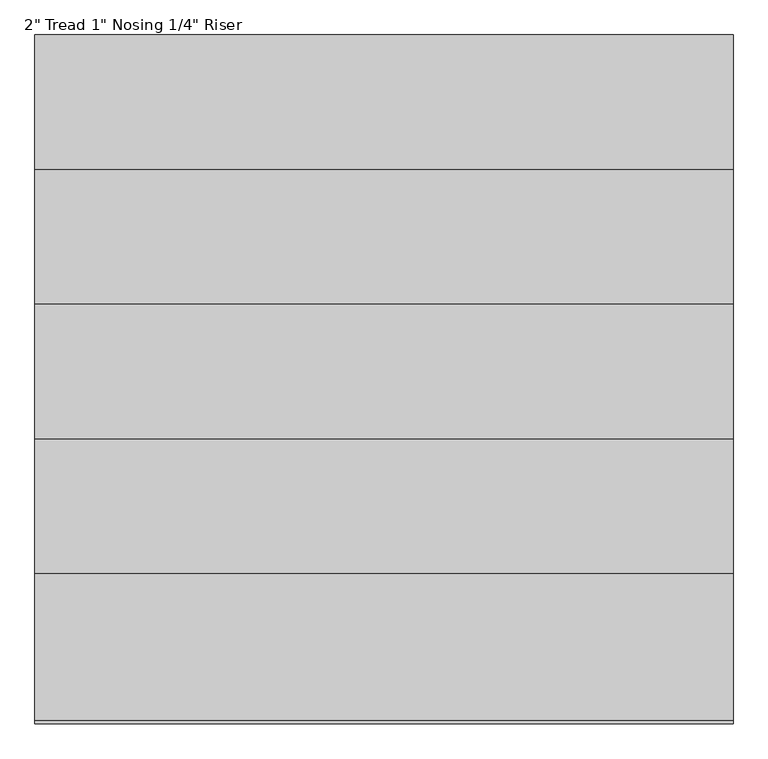
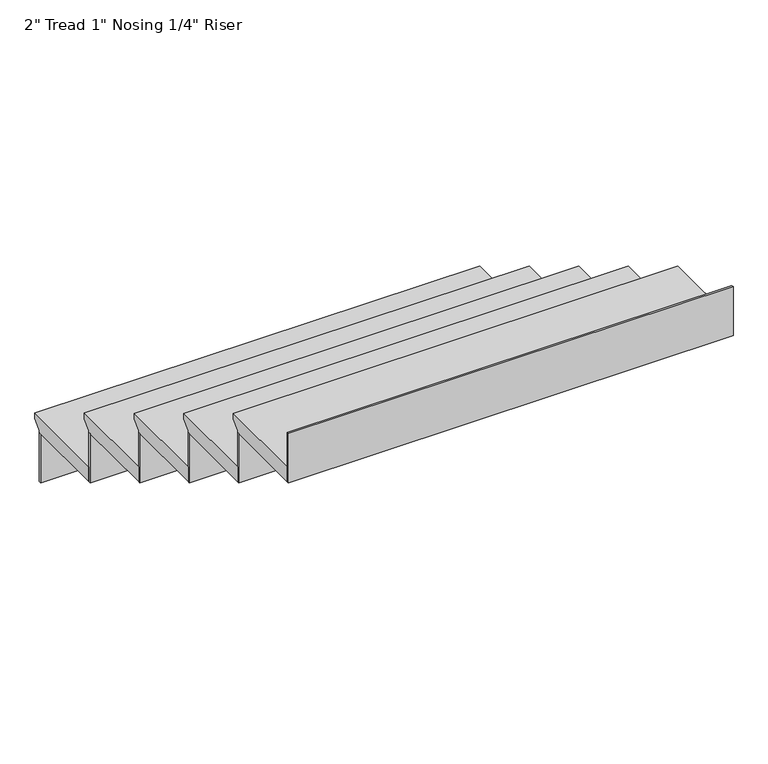
"""IFC4 building model written with IfcOpenShell, lengths in millimetres: stair flight geometry."""

from ifc_helpers import new_model, si_unit, frame, origin, place, context, project, spatial, polyline, outline, extrude, source, transform, mapped, element, save


def stair_flight_724757b1(model_context):
    return source(origin(), model_context, "Body", "SweptSolid", [
        extrude(outline(polyline([(3133.6258877, 2201.3333333), (3438.4258877, 2201.3333333), (3438.4258877, 2182.2833333), (3413.0258877, 2156.8833333), (3413.0258877, 2150.5333333), (3133.6258877, 2150.5333333), (3133.6258877, 2201.3333333)])), frame((-16853.0480019, 0.0, 0.0), z_axis=(1.0, 0.0, 0.0), x_axis=(0.0, 1.0, 0.0)), (0.0, 0.0, 1.0), 1447.8),
        extrude(outline(polyline([(-16853.0480019, 3406.6758877), (-16853.0480019, 3413.0258877), (-15405.2480019, 3413.0258877), (-15405.2480019, 3406.6758877), (-16853.0480019, 3406.6758877)])), frame((0.0, 0.0, 1981.2), z_axis=(0.0, 0.0, 1.0), x_axis=(1.0, 0.0, 0.0)), (0.0, 0.0, 1.0), 169.3333333),
        extrude(outline(polyline([(-16853.0480019, 3127.2758877), (-16853.0480019, 3133.6258877), (-15405.2480019, 3133.6258877), (-15405.2480019, 3127.2758877), (-16853.0480019, 3127.2758877)])), frame((0.0, 0.0, 2150.5333333), z_axis=(0.0, 0.0, 1.0), x_axis=(1.0, 0.0, 0.0)), (0.0, 0.0, 1.0), 169.3333333),
        extrude(outline(polyline([(2854.2258877, 2370.6666667), (3159.0258877, 2370.6666667), (3159.0258877, 2351.6166667), (3133.6258877, 2326.2166667), (3133.6258877, 2319.8666667), (2854.2258877, 2319.8666667), (2854.2258877, 2370.6666667)])), frame((-16853.0480019, 0.0, 0.0), z_axis=(1.0, 0.0, 0.0), x_axis=(0.0, 1.0, 0.0)), (0.0, 0.0, 1.0), 1447.8),
        extrude(outline(polyline([(-16853.0480019, 2847.8758877), (-16853.0480019, 2854.2258877), (-15405.2480019, 2854.2258877), (-15405.2480019, 2847.8758877), (-16853.0480019, 2847.8758877)])), frame((0.0, 0.0, 2319.8666667), z_axis=(0.0, 0.0, 1.0), x_axis=(1.0, 0.0, 0.0)), (0.0, 0.0, 1.0), 169.3333333),
        extrude(outline(polyline([(2574.8258877, 2540.0), (2879.6258877, 2540.0), (2879.6258877, 2520.95), (2854.2258877, 2495.55), (2854.2258877, 2489.2), (2574.8258877, 2489.2), (2574.8258877, 2540.0)])), frame((-16853.0480019, 0.0, 0.0), z_axis=(1.0, 0.0, 0.0), x_axis=(0.0, 1.0, 0.0)), (0.0, 0.0, 1.0), 1447.8),
        extrude(outline(polyline([(-16853.0480019, 2568.4758877), (-16853.0480019, 2574.8258877), (-15405.2480019, 2574.8258877), (-15405.2480019, 2568.4758877), (-16853.0480019, 2568.4758877)])), frame((0.0, 0.0, 2489.2), z_axis=(0.0, 0.0, 1.0), x_axis=(1.0, 0.0, 0.0)), (0.0, 0.0, 1.0), 169.3333333),
        extrude(outline(polyline([(2295.4258877, 2709.3333333), (2600.2258877, 2709.3333333), (2600.2258877, 2690.2833333), (2574.8258877, 2664.8833333), (2574.8258877, 2658.5333333), (2295.4258877, 2658.5333333), (2295.4258877, 2709.3333333)])), frame((-16853.0480019, 0.0, 0.0), z_axis=(1.0, 0.0, 0.0), x_axis=(0.0, 1.0, 0.0)), (0.0, 0.0, 1.0), 1447.8),
        extrude(outline(polyline([(-16853.0480019, 2289.0758877), (-16853.0480019, 2295.4258877), (-15405.2480019, 2295.4258877), (-15405.2480019, 2289.0758877), (-16853.0480019, 2289.0758877)])), frame((0.0, 0.0, 2658.5333333), z_axis=(0.0, 0.0, 1.0), x_axis=(1.0, 0.0, 0.0)), (0.0, 0.0, 1.0), 169.3333333),
        extrude(outline(polyline([(-16853.0480019, 2009.6758877), (-16853.0480019, 2016.0258877), (-15405.2480019, 2016.0258877), (-15405.2480019, 2009.6758877), (-16853.0480019, 2009.6758877)])), frame((0.0, 0.0, 2827.8666667), z_axis=(0.0, 0.0, 1.0), x_axis=(1.0, 0.0, 0.0)), (0.0, 0.0, 1.0), 169.3333333),
        extrude(outline(polyline([(2016.0258877, 2878.6666667), (2320.8258877, 2878.6666667), (2320.8258877, 2859.6166667), (2295.4258877, 2834.2166667), (2295.4258877, 2827.8666667), (2016.0258877, 2827.8666667), (2016.0258877, 2878.6666667)])), frame((-16853.0480019, 0.0, 0.0), z_axis=(1.0, 0.0, 0.0), x_axis=(0.0, 1.0, 0.0)), (0.0, 0.0, 1.0), 1447.8),
    ])


if __name__ == "__main__":
    model = new_model("IFC4")
    model_context = context("Model", 3, world=origin())
    ifc_project = project(units=[si_unit("LENGTHUNIT", "METRE", prefix="MILLI")], contexts=[model_context])
    site = spatial("IfcSite", under=ifc_project)
    building = spatial("IfcBuilding", under=site)
    placement = place(None, origin())
    stair_flight_shape = stair_flight_724757b1(model_context)
    element("IfcStairFlight", 1, ObjectType="2\" Tread 1\" Nosing 1/4\" Riser", at=placement, inside=building, context=model_context, shape_type="MappedRepresentation", body=[
        mapped(stair_flight_shape, transform((0.0, 0.0, 0.0), x_axis=(1.0, 0.0, 0.0), y_axis=(0.0, 1.0, 0.0), z_axis=(0.0, 0.0, 1.0))),
    ])
    save(model, "model.ifc")
